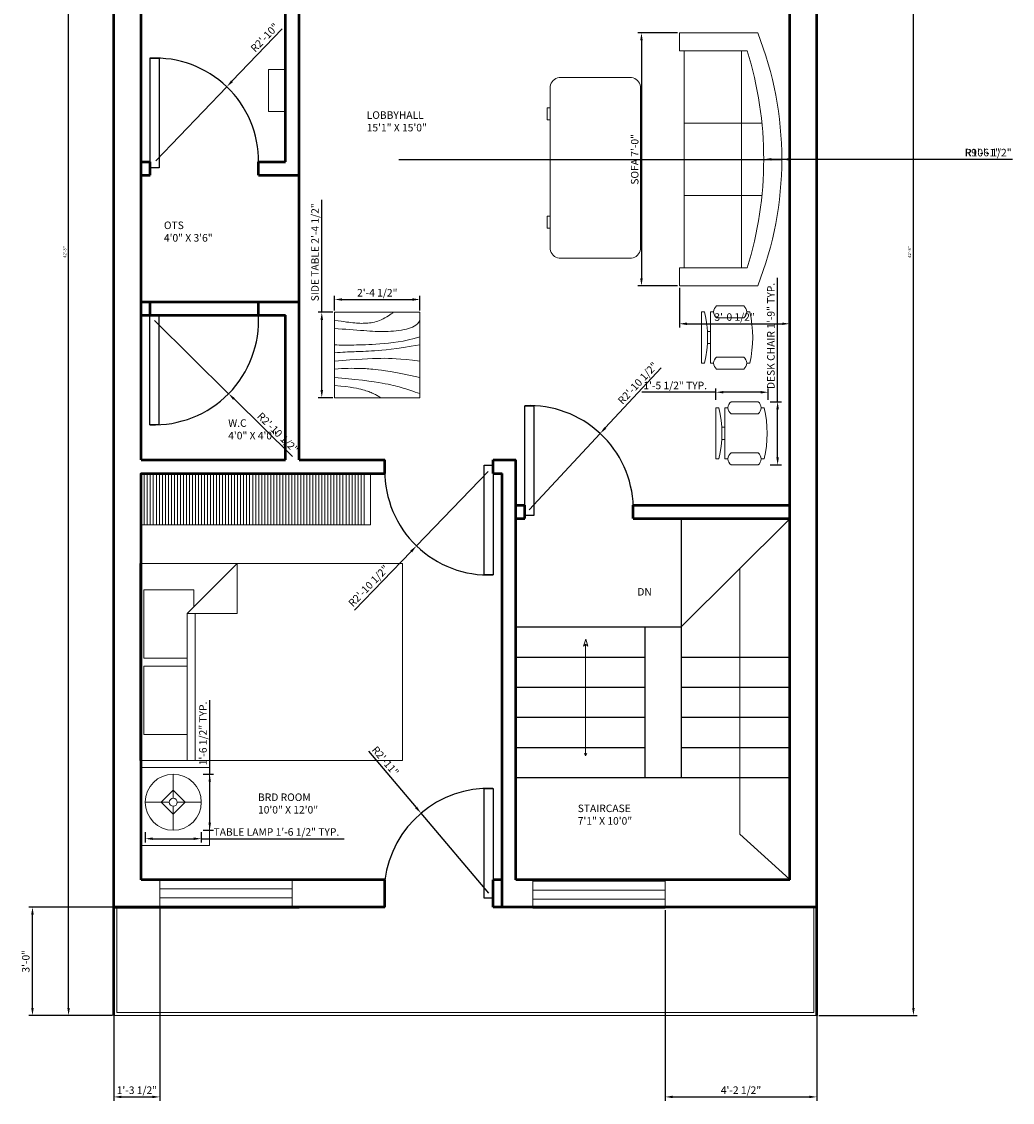
# Model space of a CAD drawing. Units: inches. Extents: x 210 to 950, y 0 to 561.
# Tile 4 of 5: x 621 to 950, y 8 to 366. Entities that reach past the tile are written whole.
import ezdxf

# ---------------------------------------------------------------- set-up
doc = ezdxf.new("R2010")
doc.units = ezdxf.units.IN
for name, color, linetype, lineweight in [('A-ANNO-DIMS', 2, 'Continuous', 18), ('A-ANNO-SYMB', 7, 'Continuous', 18), ('A-ANNO-TEXT', 7, 'Continuous', 18), ('A-AREA-IDEN', 7, 'Continuous', 18), ('A-DOOR', 4, 'Continuous', 25), ('A-FLOR-CASE', 8, 'Continuous', 20), ('A-FLOR-FIXT', 9, 'Continuous', 18), ('A-FLOR-HRAL', 7, 'Continuous', 18), ('A-FLOR-STRS', 7, 'Continuous', 25), ('A-FURN', 8, 'Continuous', 18), ('A-FURN-PATT', 9, 'Continuous', 13), ('A-GLAZ', 4, 'Continuous', 20), ('A-WALL', 7, 'Continuous', 50)]:
    doc.layers.add(name, color=color, linetype=linetype, lineweight=lineweight)
doc.styles.get("Standard").update_dxf_attribs({"font": 'arial.ttf'})
doc.dimstyles.new('ISO-25', dxfattribs={"dimtxt": 2.5, "dimasz": 2.5, "dimexe": 1.25, "dimexo": 0.625, "dimtad": 1, "dimtxsty": 'Standard', "dimcen": 2.5, "dimadec": 0, "dimazin": 0, "dimtfac": 1, "dimtmove": 0, "dimatfit": 3, "dimfxl": 1, "dimarcsym": 0})

# ---------------------------------------------------------------- blocks, each defined once
blk = doc.blocks.new('Bed - Queen')
for p, q in [((0, -80.00003), (0, 0)), ((0, 0), (59.99999, 0)), ((59.99999, 0), (59.99999, -80.00003)), ((7.99999, -1.2), (28.79998, -1.2)), ((7.99999, -14.4), (7.99999, -1.2)), ((28.79998, -1.2), (28.79998, -14.4)), ((31.19999, -1.2), (51.99999, -1.2)), ((31.19999, -14.4), (31.19999, -1.2)), ((51.99999, -1.2), (51.99999, -16.4)), ((0, -14.4), (44.8, -14.4)), ((59.99999, -29.6), (44.8, -14.4)), ((44.8, -14.4), (44.8, -29.6)), ((51.99999, -16.4), (46.79936, -16.4)), ((44.8, -16.8), (0, -16.8)), ((44.8, -29.6), (59.99999, -29.6)), ((59.99999, -80.00003), (0, -80.00003))]:
    blk.add_line(p, q)
blk = doc.blocks.new('Lamp - Table')
for p, q in [((0, 7), (0, 1)), ((0, 3), (-3, 0)), ((3, 0), (0, 3)), ((-1, 0), (-7, 0)), ((-3, 0), (0, -3)), ((0, -3), (3, 0)), ((1, 0), (7, 0)), ((0, -1), (0, -7))]:
    blk.add_line(p, q)
for radius in [7, 1]:
    blk.add_circle((0, 0), radius)
blk = doc.blocks.new('Sofa - Roundback 7 ft.')
for p, q in [((-12.00002, -32.4421), (-12.00003, -6.5971)), ((11.99997, -32.4421), (11.99998, -6.5971)), ((-36.000027, -34), (-36.000027, -11.4696)), ((-35.999844, -13.3819), (35.9998, -13.3819)), ((35.99998, -34), (35.99998, -11.4696)), ((-36.000027, -32.4421), (35.99998, -32.4421))]:
    blk.add_line(p, q)
for points in [[(-36.000027, -34), (-42.000027, -34), (-42.000027, -8)], [(41.99998, -8), (41.99998, -34), (35.99998, -34)]]:
    blk.add_lwpolyline(points)
for centre, radius, start, end in [((0, -114.25), 114.25, 68.43141, 111.5686), ((-0.00001, -127.1968), 121.1968, 72.72033, 107.2797)]:
    blk.add_arc(centre, radius, start, end)
blk = doc.blocks.new('Chair - Desk')
for p, q in [((-8.5, 0), (-8.5, -1)), ((-8.5, 0), (8.5, 0)), ((8.5, 0), (8.5, -1)), ((-8.5, -3), (-8.5, -4)), ((-8.5, -3), (8.5, -3)), ((-2, -3), (-2, -1.9355)), ((2, -1.9576), (2, -3)), ((8.5, -3), (8.5, -4)), ((-10.5, -5), (-10.5, -14)), ((-6.5, -14), (-6.5, -5)), ((6.5, -5), (6.5, -14)), ((10.5, -14), (10.5, -5)), ((-8.5, -15), (-8.5, -16)), ((8.5, -15), (8.5, -16))]:
    blk.add_line(p, q)
for centre, radius, start, end in [((0, 34.625), 36.625, 256.5803, 283.4197), ((-8.5, -6.5), 2.5, 36.8699, 143.1301), ((8.5, -6.5), 2.5, 36.8699, 143.1301), ((-8.5, -12.5), 2.5, 216.8699, 323.1301), ((8.5, -12.5), 2.5, 216.8699, 323.1301), ((0, 19.625), 36.625, 256.5803, 283.4197)]:
    blk.add_arc(centre, radius, start, end)
blk = doc.blocks.new('Desk - 30 x 60 in.')
for p, q in [((-26.999995, 0), (26.999995, 0)), ((-29.999995, -27), (-29.999995, -3)), ((29.999995, -3), (29.999995, -27)), ((26.999995, -30), (-26.999995, -30)), ((-20.000005, -30), (-20.000005, -31)), ((-20.000005, -31), (-16.000005, -31)), ((-16.000005, -31), (-16.000005, -30)), ((15.999995, -31), (15.999995, -30)), ((19.999995, -31), (15.999995, -31)), ((19.999995, -30), (19.999995, -31))]:
    blk.add_line(p, q)
for centre, start, end in [((-26.499995, -3.5), 98.1301, 171.8699), ((26.499995, -3.5), 8.130102, 81.8699), ((-26.499995, -26.5), 188.1301, 261.8699), ((26.499995, -26.5), 278.1301, 351.8699)]:
    blk.add_arc(centre, 3.535534, start, end)
blk = doc.blocks.new('Table - Square Woodgrain 42 x 42 in.')
blk.add_line((0, -42), (42, -42))
for points in [[(0, -4), (1.704, -4.2172), (3.2358, -4.4188), (4.615, -4.604), (5.8615, -4.7721), (6.9951, -4.9224), (8.0357, -5.0541), (9.0031, -5.1667), (9.9171, -5.2594), (10.7951, -5.3316), (11.6445, -5.3836), (12.4702, -5.4157), (13.277, -5.4283), (14.0698, -5.4217), (14.8535, -5.3964), (15.6331, -5.3526), (16.4133, -5.2908), (17.1986, -5.2103), (17.9913, -5.1062), (18.793, -4.9727), (19.6056, -4.8038), (20.4307, -4.5937), (21.2701, -4.3365), (22.1256, -4.0262), (22.9989, -3.6571), (23.888, -3.2272), (24.7756, -2.7516), (25.6408, -2.2491), (26.4624, -1.7387), (27.2195, -1.2395), (27.891, -0.7703), (28.456, -0.3501), (28.8934, 0.002)], [(0, -42), (0, 0), (42, 0), (42, -42)], [(0, -8), (1.8203, -8.1001), (3.6741, -8.2149), (5.5411, -8.3408), (7.4011, -8.4741), (9.2339, -8.6112), (11.0193, -8.7484), (12.7371, -8.8821), (14.3671, -9.0086), (15.8954, -9.1246), (17.3337, -9.2278), (18.6997, -9.3159), (20.0116, -9.387), (21.2871, -9.4389), (22.5442, -9.4696), (23.8008, -9.477), (25.0749, -9.459), (26.3791, -9.4137), (27.7049, -9.3403), (29.0383, -9.2382), (30.3655, -9.1068), (31.6728, -8.9455), (32.9461, -8.7535), (34.1717, -8.5304), (35.3358, -8.2756), (36.4268, -7.9863), (37.443, -7.6521), (38.3849, -7.2603), (39.253, -6.7986), (40.048, -6.2542), (40.7705, -5.6147), (41.421, -4.8674), (42, -4)], [(42, -12), (39.1784, -12.8621), (36.4519, -13.5654), (33.8246, -14.1294), (31.3004, -14.5731), (28.8832, -14.9161), (26.577, -15.1775), (24.3858, -15.3768), (22.3136, -15.5332), (20.3622, -15.6632), (18.5254, -15.7718), (16.7947, -15.8612), (15.1618, -15.9338), (13.6183, -15.9916), (12.1558, -16.0369), (10.7659, -16.0718), (9.4403, -16.0987), (8.1703, -16.1191), (6.9461, -16.1325), (5.7577, -16.1377), (4.595, -16.1335), (3.4479, -16.1188), (2.3064, -16.0924), (1.1604, -16.0532), (0, -16)], [(42, -16), (37.6529, -16.7365), (33.8802, -17.329), (30.6179, -17.7961), (27.8015, -18.1561), (25.3668, -18.4275), (23.2497, -18.6288), (21.3859, -18.7785), (19.7111, -18.8949), (18.1693, -18.9939), (16.7375, -19.0795), (15.401, -19.1534), (14.1449, -19.217), (12.9544, -19.2717), (11.8148, -19.3191), (10.7113, -19.3606), (9.6291, -19.3976), (8.5534, -19.4323), (7.47, -19.4689), (6.3643, -19.5122), (5.222, -19.5672), (4.0288, -19.6386), (2.7703, -19.7313), (1.4321, -19.8501), (0, -20)], [(0, -24), (3.9243, -23.6805), (7.4766, -23.4138), (10.6891, -23.1954), (13.5943, -23.0205), (16.2247, -22.8847), (18.6125, -22.7832), (20.7903, -22.7116), (22.7903, -22.6651), (24.6563, -22.642), (26.4764, -22.6507), (28.35, -22.7024), (30.3766, -22.8084), (32.6555, -22.98), (35.2861, -23.2283), (38.3678, -23.5645), (42, -24)], [(42, -32), (37.392, -31.017), (33.4585, -30.2231), (30.1291, -29.5949), (27.3334, -29.109), (25.0009, -28.742), (23.0612, -28.4707), (21.4439, -28.2716), (20.0786, -28.1215), (18.8998, -28.0002), (17.8609, -27.9014), (16.9206, -27.8219), (16.0371, -27.7588), (15.1691, -27.709), (14.2748, -27.6693), (13.3128, -27.6368), (12.2415, -27.6083), (11.0295, -27.5824), (9.6867, -27.5643), (8.233, -27.5608), (6.6884, -27.5787), (5.0728, -27.6248), (3.4062, -27.7058), (1.7086, -27.8286), (0, -28)], [(0, -32), (5.4026, -32.5358), (9.9494, -33.019), (13.7424, -33.4553), (16.8834, -33.8505), (19.4743, -34.2106), (21.6171, -34.5413), (23.4136, -34.8486), (24.9657, -35.1382), (26.3614, -35.4156), (27.6332, -35.6841), (28.7995, -35.9467), (29.8788, -36.2064), (30.8897, -36.4661), (31.8507, -36.7288), (32.7802, -36.9973), (33.6968, -37.2747), (34.6175, -37.5635), (35.5531, -37.8651), (36.5128, -38.1805), (37.506, -38.5108), (38.5421, -38.8568), (39.6302, -39.2197), (40.7797, -39.6004), (42, -40)], [(0, -36), (3.0098, -36.2857), (5.5354, -36.5643), (7.6368, -36.8359), (9.374, -37.1009), (10.807, -37.3597), (11.9957, -37.6126), (13.0002, -37.8599), (13.8804, -38.102), (14.6874, -38.3393), (15.4365, -38.5729), (16.1338, -38.8041), (16.7858, -39.0341), (17.3987, -39.264), (17.9787, -39.4952), (18.5322, -39.7288), (19.0655, -39.9662), (19.5832, -40.2081), (20.0842, -40.4544), (20.5657, -40.7046), (21.0249, -40.9581), (21.459, -41.2144), (21.8653, -41.4731), (22.2409, -41.7335), (22.5831, -41.9951)]]:
    blk.add_lwpolyline(points)
blk = doc.blocks.new('*D17')
at = {"layer": 'A-ANNO-DIMS', "color": 0, "lineweight": -2, "transparency": 16777216}
for p, q in [((651.28, 543.37), (635.61, 543.37)), ((636.86, 38.87), (636.86, 540.87)), ((651.28, 36.37), (635.61, 36.37))]:
    blk.add_line(p, q, dxfattribs=at)
at = {"layer": 'A-ANNO-DIMS', "color": 0, "transparency": 16777216}
for points in [[(636.44, 540.87), (637.27, 540.87), (636.86, 543.37)], [(636.44, 38.87), (637.27, 38.87), (636.86, 36.37)]]:
    blk.add_solid(points, dxfattribs=at)
at = {"layer": 'Defpoints', "color": 0, "transparency": 16777216}
for p in [(636.86, 543.37), (651.91, 543.37), (651.91, 36.37)]:
    blk.add_point(p, dxfattribs=at)
at = {"layer": 'A-ANNO-DIMS', "color": 0, "transparency": 16777216, "insert": (635.72, 289.87), "char_height": 1, "attachment_point": 5, "rotation": 90}
blk.add_mtext('42\'-3"', dxfattribs=at)
blk = doc.blocks.new('*D19')
at = {"layer": 'A-ANNO-DIMS', "color": 0, "lineweight": -2, "transparency": 16777216}
for p, q in [((886.03, 543.37), (918.72, 543.37)), ((917.47, 38.87), (917.47, 540.87)), ((886.03, 36.37), (918.72, 36.37))]:
    blk.add_line(p, q, dxfattribs=at)
at = {"layer": 'A-ANNO-DIMS', "color": 0, "transparency": 16777216}
for points in [[(917.05, 540.87), (917.89, 540.87), (917.47, 543.37)], [(917.05, 38.87), (917.89, 38.87), (917.47, 36.37)]]:
    blk.add_solid(points, dxfattribs=at)
at = {"layer": 'Defpoints', "color": 0, "transparency": 16777216}
for p in [(885.41, 543.37), (917.47, 543.37), (885.41, 36.37)]:
    blk.add_point(p, dxfattribs=at)
at = {"layer": 'A-ANNO-DIMS', "color": 0, "transparency": 16777216, "insert": (916.33, 289.87), "char_height": 1, "attachment_point": 5, "rotation": 90}
blk.add_mtext('42\'-3"', dxfattribs=at)
blk = doc.blocks.new('WIN-44IN-DEEP-FRAME')
for p, q in [((0, 0), (0, 9)), ((0, 9), (43.89, 9)), ((43.89, 9), (43.89, 0)), ((43.89, 6), (0, 6)), ((0, 3), (43.89, 3)), ((43.89, 0), (0, 0))]:
    blk.add_line(p, q)
blk = doc.blocks.new('DOOR-LEAF-36IN')
blk.add_lwpolyline([(0, 0), (0, -2.99), (-36.41, -2.99), (-36.41, 0)], close=True)
blk = doc.blocks.new('*D26')
at = {"layer": 'A-ANNO-DIMS', "color": 0, "lineweight": -2, "transparency": 16777216}
for p, q in [((662.31, 97.23), (662.31, 93.81)), ((680.94, 97.23), (680.94, 93.81)), ((664.81, 95.06), (678.44, 95.06)), ((680.94, 95.06), (728.34, 95.06))]:
    blk.add_line(p, q, dxfattribs=at)
at = {"layer": 'A-ANNO-DIMS', "color": 0, "transparency": 16777216}
for points in [[(664.81, 95.48), (664.81, 94.64), (662.31, 95.06)], [(678.44, 95.48), (678.44, 94.64), (680.94, 95.06)]]:
    blk.add_solid(points, dxfattribs=at)
at = {"layer": 'Defpoints', "color": 0, "transparency": 16777216}
for p in [(662.31, 97.85), (680.94, 97.85), (680.94, 95.06)]:
    blk.add_point(p, dxfattribs=at)
at = {"layer": 'A-ANNO-DIMS', "color": 0, "transparency": 16777216, "insert": (705.89, 96.98), "char_height": 2.5, "attachment_point": 5}
blk.add_mtext('TABLE LAMP 1\'-6 1/2" TYP.', dxfattribs=at)
blk = doc.blocks.new('*D27')
at = {"layer": 'A-ANNO-DIMS', "color": 0, "lineweight": -2, "transparency": 16777216}
for p, q in [((683.74, 116.48), (683.74, 141.06)), ((681.57, 116.48), (684.99, 116.48)), ((683.74, 100.35), (683.74, 113.98)), ((681.57, 97.85), (684.99, 97.85))]:
    blk.add_line(p, q, dxfattribs=at)
at = {"layer": 'A-ANNO-DIMS', "color": 0, "transparency": 16777216}
for points in [[(683.32, 113.98), (684.15, 113.98), (683.74, 116.48)], [(683.32, 100.35), (684.15, 100.35), (683.74, 97.85)]]:
    blk.add_solid(points, dxfattribs=at)
at = {"layer": 'Defpoints', "color": 0, "transparency": 16777216}
for p in [(680.94, 116.48), (683.74, 116.48), (680.94, 97.85)]:
    blk.add_point(p, dxfattribs=at)
at = {"layer": 'A-ANNO-DIMS', "color": 0, "transparency": 16777216, "insert": (681.82, 130.02), "char_height": 2.5, "attachment_point": 5, "rotation": 90}
blk.add_mtext('1\'-6 1/2" TYP.', dxfattribs=at)
blk = doc.blocks.new('*D28')
at = {"layer": 'A-ANNO-DIMS', "color": 0, "lineweight": -2, "transparency": 16777216}
for p, q in [((872.36, 240.17), (872.36, 281.35)), ((869.84, 240.17), (873.61, 240.17)), ((872.36, 221.67), (872.36, 237.67)), ((869.84, 219.17), (873.61, 219.17))]:
    blk.add_line(p, q, dxfattribs=at)
at = {"layer": 'A-ANNO-DIMS', "color": 0, "transparency": 16777216}
for points in [[(871.95, 237.67), (872.78, 237.67), (872.36, 240.17)], [(871.95, 221.67), (872.78, 221.67), (872.36, 219.17)]]:
    blk.add_solid(points, dxfattribs=at)
at = {"layer": 'Defpoints', "color": 0, "transparency": 16777216}
for p in [(869.21, 240.17), (872.36, 240.17), (869.21, 219.17)]:
    blk.add_point(p, dxfattribs=at)
at = {"layer": 'A-ANNO-DIMS', "color": 0, "transparency": 16777216, "insert": (870.45, 262.01), "char_height": 2.5, "attachment_point": 5, "rotation": 90}
blk.add_mtext('DESK CHAIR 1\'-9" TYP.', dxfattribs=at)
blk = doc.blocks.new('*D29')
at = {"layer": 'A-ANNO-DIMS', "color": 0, "lineweight": -2, "transparency": 16777216}
for p, q in [((851.88, 240.79), (851.88, 244.57)), ((869.21, 240.79), (869.21, 244.57)), ((851.88, 243.32), (827.3, 243.32)), ((866.71, 243.32), (854.38, 243.32))]:
    blk.add_line(p, q, dxfattribs=at)
at = {"layer": 'A-ANNO-DIMS', "color": 0, "transparency": 16777216}
for points in [[(854.38, 243.73), (854.38, 242.9), (851.88, 243.32)], [(866.71, 243.73), (866.71, 242.9), (869.21, 243.32)]]:
    blk.add_solid(points, dxfattribs=at)
at = {"layer": 'Defpoints', "color": 0, "transparency": 16777216}
for p in [(851.88, 243.32), (851.88, 240.17), (869.21, 240.17)]:
    blk.add_point(p, dxfattribs=at)
at = {"layer": 'A-ANNO-DIMS', "color": 0, "transparency": 16777216, "insert": (838.34, 245.24), "char_height": 2.5, "attachment_point": 5}
blk.add_mtext('1\'-5 1/2" TYP.', dxfattribs=at)
blk = doc.blocks.new('*D34')
at = {"layer": 'A-ANNO-DIMS', "color": 0, "lineweight": -2, "transparency": 16777216}
for p, q in [((720.95, 269.86), (720.95, 307.23)), ((724.58, 269.86), (719.7, 269.86)), ((720.95, 244.01), (720.95, 267.36)), ((724.58, 241.51), (719.7, 241.51))]:
    blk.add_line(p, q, dxfattribs=at)
at = {"layer": 'A-ANNO-DIMS', "color": 0, "transparency": 16777216}
for points in [[(720.53, 267.36), (721.37, 267.36), (720.95, 269.86)], [(720.53, 244.01), (721.37, 244.01), (720.95, 241.51)]]:
    blk.add_solid(points, dxfattribs=at)
at = {"layer": 'Defpoints', "color": 0, "transparency": 16777216}
for p in [(720.95, 269.86), (725.2, 269.86), (725.2, 241.51)]:
    blk.add_point(p, dxfattribs=at)
at = {"layer": 'A-ANNO-DIMS', "color": 0, "transparency": 16777216, "insert": (719.03, 289.79), "char_height": 2.5, "attachment_point": 5, "rotation": 90}
blk.add_mtext('SIDE TABLE 2\'-4 1/2"', dxfattribs=at)
blk = doc.blocks.new('*D35')
at = {"layer": 'A-ANNO-DIMS', "color": 0, "lineweight": -2, "transparency": 16777216}
for p, q in [((725.2, 270.49), (725.2, 275.36)), ((727.7, 274.11), (751.05, 274.11)), ((753.55, 270.49), (753.55, 275.36))]:
    blk.add_line(p, q, dxfattribs=at)
at = {"layer": 'A-ANNO-DIMS', "color": 0, "transparency": 16777216}
for points in [[(727.7, 274.53), (727.7, 273.7), (725.2, 274.11)], [(751.05, 274.53), (751.05, 273.7), (753.55, 274.11)]]:
    blk.add_solid(points, dxfattribs=at)
at = {"layer": 'Defpoints', "color": 0, "transparency": 16777216}
for p in [(753.55, 274.11), (725.2, 269.86), (753.55, 269.86)]:
    blk.add_point(p, dxfattribs=at)
at = {"layer": 'A-ANNO-DIMS', "color": 0, "transparency": 16777216, "insert": (739.38, 276.03), "char_height": 2.5, "attachment_point": 5}
blk.add_mtext('2\'-4 1/2"', dxfattribs=at)
blk = doc.blocks.new('*D40')
at = {"layer": 'A-ANNO-DIMS', "color": 0, "lineweight": -2, "transparency": 16777216}
for p, q in [((839.11, 362.65), (825.89, 362.65)), ((827.14, 360.15), (827.14, 281.15)), ((839.11, 278.65), (825.89, 278.65))]:
    blk.add_line(p, q, dxfattribs=at)
at = {"layer": 'A-ANNO-DIMS', "color": 0, "transparency": 16777216}
for points in [[(826.72, 360.15), (827.55, 360.15), (827.14, 362.65)], [(826.72, 281.15), (827.55, 281.15), (827.14, 278.65)]]:
    blk.add_solid(points, dxfattribs=at)
at = {"layer": 'Defpoints', "color": 0, "transparency": 16777216}
for p in [(839.74, 362.65), (827.14, 278.65), (839.74, 278.65)]:
    blk.add_point(p, dxfattribs=at)
at = {"layer": 'A-ANNO-DIMS', "color": 0, "transparency": 16777216, "insert": (825.22, 320.65), "char_height": 2.5, "attachment_point": 5, "rotation": 90}
blk.add_mtext('SOFA 7\'-0"', dxfattribs=at)
blk = doc.blocks.new('*D41')
at = {"layer": 'A-ANNO-DIMS', "color": 0, "lineweight": -2, "transparency": 16777216}
for p, q in [((839.74, 278.03), (839.74, 264.8)), ((876.4, 278.03), (876.4, 264.8)), ((842.24, 266.05), (873.9, 266.05))]:
    blk.add_line(p, q, dxfattribs=at)
at = {"layer": 'A-ANNO-DIMS', "color": 0, "transparency": 16777216}
for points in [[(842.24, 266.47), (842.24, 265.64), (839.74, 266.05)], [(873.9, 266.47), (873.9, 265.64), (876.4, 266.05)]]:
    blk.add_solid(points, dxfattribs=at)
at = {"layer": 'Defpoints', "color": 0, "transparency": 16777216}
for p in [(839.74, 278.65), (876.4, 278.65), (876.4, 266.05)]:
    blk.add_point(p, dxfattribs=at)
at = {"layer": 'A-ANNO-DIMS', "color": 0, "transparency": 16777216, "insert": (858.07, 267.97), "char_height": 2.5, "attachment_point": 5}
blk.add_mtext('3\'-0 1/2"', dxfattribs=at)
blk = doc.blocks.new('*D48')
at = {"layer": 'A-ANNO-DIMS', "color": 0, "lineweight": -2, "transparency": 16777216}
for p, q in [((651.28, 72.37), (623.61, 72.37)), ((624.86, 38.87), (624.86, 69.87)), ((651.28, 36.37), (623.61, 36.37))]:
    blk.add_line(p, q, dxfattribs=at)
at = {"layer": 'A-ANNO-DIMS', "color": 0, "transparency": 16777216}
for points in [[(624.44, 69.87), (625.27, 69.87), (624.86, 72.37)], [(624.44, 38.87), (625.27, 38.87), (624.86, 36.37)]]:
    blk.add_solid(points, dxfattribs=at)
at = {"layer": 'Defpoints', "color": 0, "transparency": 16777216}
for p in [(624.86, 72.37), (651.91, 72.37), (651.91, 36.37)]:
    blk.add_point(p, dxfattribs=at)
at = {"layer": 'A-ANNO-DIMS', "color": 0, "transparency": 16777216, "insert": (622.96, 54.37), "char_height": 2.5, "attachment_point": 5, "rotation": 90}
blk.add_mtext('3\'-0"', dxfattribs=at)
blk = doc.blocks.new('*D50')
at = {"layer": 'A-ANNO-DIMS', "color": 0, "lineweight": -2, "transparency": 16777216}
for p, q in [((651.91, 71.74), (651.91, 8.07)), ((667.18, 71.76), (667.18, 8.07)), ((654.41, 9.32), (664.68, 9.32))]:
    blk.add_line(p, q, dxfattribs=at)
at = {"layer": 'A-ANNO-DIMS', "color": 0, "transparency": 16777216}
for points in [[(654.41, 9.73), (654.41, 8.9), (651.91, 9.32)], [(664.68, 9.73), (664.68, 8.9), (667.18, 9.32)]]:
    blk.add_solid(points, dxfattribs=at)
at = {"layer": 'Defpoints', "color": 0, "transparency": 16777216}
for p in [(651.91, 72.37), (667.18, 72.39), (667.18, 9.32)]:
    blk.add_point(p, dxfattribs=at)
at = {"layer": 'A-ANNO-DIMS', "color": 0, "transparency": 16777216, "insert": (659.54, 11.23), "char_height": 2.5, "attachment_point": 5}
blk.add_mtext('1\'-3 1/2"', dxfattribs=at)
blk = doc.blocks.new('*D51')
at = {"layer": 'A-ANNO-DIMS', "color": 0, "lineweight": -2, "transparency": 16777216}
for p, q in [((835, 71.37), (835, 8.07)), ((885.41, 71.74), (885.41, 8.07)), ((837.5, 9.32), (882.91, 9.32))]:
    blk.add_line(p, q, dxfattribs=at)
at = {"layer": 'A-ANNO-DIMS', "color": 0, "transparency": 16777216}
for points in [[(837.5, 9.73), (837.5, 8.9), (835, 9.32)], [(882.91, 9.73), (882.91, 8.9), (885.41, 9.32)]]:
    blk.add_solid(points, dxfattribs=at)
at = {"layer": 'Defpoints', "color": 0, "transparency": 16777216}
for p in [(835, 72), (885.41, 72.37), (885.41, 9.32)]:
    blk.add_point(p, dxfattribs=at)
at = {"layer": 'A-ANNO-DIMS', "color": 0, "transparency": 16777216, "insert": (860.2, 11.23), "char_height": 2.5, "attachment_point": 5}
blk.add_mtext('4\'-2 1/2"', dxfattribs=at)
blk = doc.blocks.new('*D58')
at = {"layer": 'A-ANNO-DIMS', "color": 0, "lineweight": -2, "transparency": 16777216}
for p, q in [((736.45, 124.09), (752.31, 105.42)), ((776.45, 77), (753.92, 103.52))]:
    blk.add_line(p, q, dxfattribs=at)
at = {"layer": 'A-ANNO-DIMS', "color": 0, "transparency": 16777216}
blk.add_solid([(752.62, 105.69), (751.99, 105.15), (753.92, 103.52)], dxfattribs=at)
at = {"layer": 'Defpoints', "color": 0, "transparency": 16777216}
for p in [(753.92, 103.52), (776.45, 77)]:
    blk.add_point(p, dxfattribs=at)
at = {"layer": 'A-ANNO-DIMS', "color": 0, "transparency": 16777216, "insert": (741.84, 120.64), "char_height": 2.5, "attachment_point": 5, "rotation": 310.3522}
blk.add_mtext('R2\'-11"', dxfattribs=at)
blk = doc.blocks.new('*D59')
at = {"layer": 'A-ANNO-DIMS', "color": 0, "lineweight": -2, "transparency": 16777216}
for p, q in [((665.34, 267.11), (690.01, 242.83)), ((711.25, 221.93), (691.8, 241.08))]:
    blk.add_line(p, q, dxfattribs=at)
at = {"layer": 'A-ANNO-DIMS', "color": 0, "transparency": 16777216}
blk.add_solid([(692.09, 241.37), (691.5, 240.78), (690.01, 242.83)], dxfattribs=at)
at = {"layer": 'Defpoints', "color": 0, "transparency": 16777216}
for p in [(665.34, 267.11), (690.01, 242.83)]:
    blk.add_point(p, dxfattribs=at)
at = {"layer": 'A-ANNO-DIMS', "color": 0, "transparency": 16777216, "insert": (706.16, 229.63), "char_height": 2.5, "attachment_point": 5, "rotation": 315.4554}
blk.add_mtext('R2\'-10 1/2"', dxfattribs=at)
blk = doc.blocks.new('*D60')
at = {"layer": 'A-ANNO-DIMS', "color": 0, "lineweight": -2, "transparency": 16777216}
for p, q in [((833.69, 251.41), (815.13, 231.45)), ((789.89, 204.32), (813.42, 229.62))]:
    blk.add_line(p, q, dxfattribs=at)
at = {"layer": 'A-ANNO-DIMS', "color": 0, "transparency": 16777216}
blk.add_solid([(814.82, 231.73), (815.43, 231.17), (813.42, 229.62)], dxfattribs=at)
at = {"layer": 'Defpoints', "color": 0, "transparency": 16777216}
for p in [(813.42, 229.62), (789.89, 204.32)]:
    blk.add_point(p, dxfattribs=at)
at = {"layer": 'A-ANNO-DIMS', "color": 0, "transparency": 16777216, "insert": (826.14, 246.11), "char_height": 2.5, "attachment_point": 5, "rotation": 47.0742}
blk.add_mtext('R2\'-10 1/2"', dxfattribs=at)
blk = doc.blocks.new('*D61')
at = {"layer": 'A-ANNO-DIMS', "color": 0, "lineweight": -2, "transparency": 16777216}
for p, q in [((776.26, 217), (752.41, 192.28)), ((731.83, 170.95), (750.68, 190.48))]:
    blk.add_line(p, q, dxfattribs=at)
at = {"layer": 'A-ANNO-DIMS', "color": 0, "transparency": 16777216}
blk.add_solid([(750.38, 190.77), (750.97, 190.19), (752.41, 192.28)], dxfattribs=at)
at = {"layer": 'Defpoints', "color": 0, "transparency": 16777216}
for p in [(776.26, 217), (752.41, 192.28)]:
    blk.add_point(p, dxfattribs=at)
at = {"layer": 'A-ANNO-DIMS', "color": 0, "transparency": 16777216, "insert": (736.72, 178.78), "char_height": 2.5, "attachment_point": 5, "rotation": 46.0238}
blk.add_mtext('R2\'-10 1/2"', dxfattribs=at)
blk = doc.blocks.new('*D63')
at = {"layer": 'A-ANNO-DIMS', "color": 0, "lineweight": -2, "transparency": 16777216}
for p, q in [((707.81, 363.95), (691.13, 346.56)), ((665.79, 320.12), (689.4, 344.76))]:
    blk.add_line(p, q, dxfattribs=at)
at = {"layer": 'A-ANNO-DIMS', "color": 0, "transparency": 16777216}
blk.add_solid([(690.83, 346.85), (691.44, 346.28), (689.4, 344.76)], dxfattribs=at)
at = {"layer": 'Defpoints', "color": 0, "transparency": 16777216}
for p in [(689.4, 344.76), (665.79, 320.12)]:
    blk.add_point(p, dxfattribs=at)
at = {"layer": 'A-ANNO-DIMS', "color": 0, "transparency": 16777216, "insert": (702.2, 360.86), "char_height": 2.5, "attachment_point": 5, "rotation": 46.2105}
blk.add_mtext('R2\'-10"', dxfattribs=at)
blk = doc.blocks.new('*D67')
at = {"layer": 'A-ANNO-DIMS', "color": 0, "lineweight": -2, "transparency": 16777216}
for p, q in [((746.54, 320.65), (867.74, 320.65)), ((946.57, 320.65), (870.24, 320.65))]:
    blk.add_line(p, q, dxfattribs=at)
at = {"layer": 'A-ANNO-DIMS', "color": 0, "transparency": 16777216}
blk.add_solid([(870.24, 321.07), (870.24, 320.24), (867.74, 320.65)], dxfattribs=at)
at = {"layer": 'Defpoints', "color": 0, "transparency": 16777216}
for p in [(746.54, 320.65), (867.74, 320.65)]:
    blk.add_point(p, dxfattribs=at)
at = {"layer": 'A-ANNO-DIMS', "color": 0, "transparency": 16777216, "insert": (940.45, 322.56), "char_height": 2.5, "attachment_point": 5}
blk.add_mtext('R10\'-1"', dxfattribs=at)
blk = doc.blocks.new('*D68')
at = {"layer": 'A-ANNO-DIMS', "color": 0, "lineweight": -2, "transparency": 16777216}
for p, q in [((759.49, 320.65), (873.74, 320.65)), ((950.34, 320.65), (876.24, 320.65))]:
    blk.add_line(p, q, dxfattribs=at)
at = {"layer": 'A-ANNO-DIMS', "color": 0, "transparency": 16777216}
blk.add_solid([(876.24, 321.07), (876.24, 320.24), (873.74, 320.65)], dxfattribs=at)
at = {"layer": 'Defpoints', "color": 0, "transparency": 16777216}
for p in [(759.49, 320.65), (873.74, 320.65)]:
    blk.add_point(p, dxfattribs=at)
at = {"layer": 'A-ANNO-DIMS', "color": 0, "transparency": 16777216, "insert": (942.29, 322.57), "char_height": 2.5, "attachment_point": 5, "rotation": 0}
blk.add_mtext('R9\'-6 1/2"', dxfattribs=at)

msp = doc.modelspace()

# ---------------------------------------------------------------- hatches: boundary and pattern name
at = {"layer": 'A-FURN-PATT'}
h = msp.add_hatch(dxfattribs=at)
h.set_pattern_fill('ANSI31', color=256, scale=0.314961, angle=45, style=0)
h.paths.add_polyline_path([(660.82, 199.32), (735.38, 199.32), (735.38, 216.37), (660.82, 216.37)])

# ---------------------------------------------------------------- linework, layer by layer
at = {"layer": 'A-ANNO-SYMB'}
for p, q in [((859.81, 96.57), (859.81, 184.76)), ((808.64, 161.32), (807.84, 158.95)), ((807.84, 158.95), (808.59, 159.57)), ((808.56, 123.16), (808.56, 159.7)), ((808.56, 159.7), (809.29, 159.05)), ((809.29, 159.05), (808.64, 161.32)), ((808.54, 122.61), (808.17, 123.37)), ((808.17, 123.37), (808.56, 123.17)), ((808.94, 123.39), (808.54, 122.61)), ((808.55, 123.16), (808.94, 123.39)), ((876.27, 81.58), (859.81, 96.57))]:
    msp.add_line(p, q, dxfattribs=at)
at = {"layer": 'A-DOOR'}
for centre, radius, start, end in [((665.79, 320.12), 34.13, 359.2311, 93.1904), ((665.34, 267.11), 34.61, 267.5759, 3.336), ((789.89, 204.32), 34.55, 1.6517, 92.4945), ((776.26, 217), 34.35, 179.4037, 272.6424), ((776.45, 77), 34.8, 87.7468, 172.9571)]:
    msp.add_arc(centre, radius, start, end, dxfattribs=at)
at = {"layer": 'A-FLOR-CASE'}
msp.add_lwpolyline([(660.78, 216.43), (737.19, 216.43), (737.19, 199.29), (660.78, 199.29)], close=True, dxfattribs=at)
at = {"layer": 'A-FLOR-FIXT'}
msp.add_lwpolyline([(708.91, 350.53), (703.27, 350.53), (703.27, 336.56), (708.91, 336.56)], close=True, dxfattribs=at)
at = {"layer": 'A-FLOR-HRAL'}
for p, q in [((652.91, 37.37), (652.91, 72.37)), ((884.41, 37.37), (884.41, 72.37)), ((885.41, 36.37), (651.91, 36.37)), ((884.41, 37.37), (652.91, 37.37)), ((885.41, 36.37), (777.91, 36.37))]:
    msp.add_line(p, q, dxfattribs=at)
at = {"layer": 'A-FLOR-STRS'}
for p, q in [((840.14, 165.19), (876.28, 201.15)), ((840.41, 115.37), (840.41, 201.37)), ((785.41, 165.37), (840.41, 165.37)), ((828.41, 115.37), (828.41, 165.37)), ((785.41, 155.37), (828.41, 155.37)), ((840.41, 155.37), (876.41, 155.37)), ((785.41, 145.37), (828.41, 145.37)), ((840.41, 145.37), (876.41, 145.37)), ((785.41, 135.37), (828.41, 135.37)), ((840.41, 135.37), (876.41, 135.37)), ((785.41, 125.37), (828.41, 125.37)), ((840.41, 125.37), (876.41, 125.37)), ((785.41, 115.37), (876.41, 115.37)), ((876.27, 81.42), (862.23, 81.42))]:
    msp.add_line(p, q, dxfattribs=at)
at = {"layer": 'A-FURN'}
msp.add_lwpolyline([(660.87, 118.7), (683.71, 118.7), (683.71, 92.84), (660.87, 92.84)], close=True, dxfattribs=at)
at = {"layer": 'A-WALL'}
for p, q in [((651.91, 36.37), (651.91, 543.37)), ((885.41, 36.37), (885.41, 543.37)), ((660.91, 315.37), (660.91, 385.87)), ((708.91, 319.87), (708.91, 385.87)), ((713.41, 315.37), (713.41, 385.87)), ((713.41, 268.87), (713.41, 385.87)), ((713.41, 220.87), (713.41, 385.87)), ((876.41, 81.37), (876.41, 385.87)), ((660.91, 319.87), (663.91, 319.87)), ((663.91, 315.37), (663.91, 319.87)), ((699.91, 315.37), (699.91, 319.87)), ((699.91, 319.87), (708.91, 319.87)), ((660.91, 315.37), (663.91, 315.37)), ((660.91, 268.87), (660.91, 315.37)), ((699.91, 315.37), (713.41, 315.37)), ((660.91, 273.37), (713.41, 273.37)), ((663.91, 268.87), (663.91, 273.37)), ((699.91, 268.87), (699.91, 273.37)), ((660.91, 268.87), (708.91, 268.87)), ((660.91, 220.87), (660.91, 268.87)), ((708.91, 220.87), (708.91, 268.87)), ((660.91, 220.87), (708.91, 220.87)), ((713.41, 220.87), (741.91, 220.87)), ((741.91, 216.37), (741.91, 220.87)), ((777.91, 216.37), (777.91, 220.87)), ((777.91, 220.87), (785.41, 220.87)), ((785.41, 81.37), (785.41, 220.87)), ((660.91, 81.37), (660.91, 216.37)), ((660.91, 216.37), (741.91, 216.37)), ((777.91, 216.37), (780.91, 216.37)), ((780.91, 72.37), (780.91, 216.37)), ((785.41, 205.87), (788.41, 205.87)), ((788.41, 201.37), (788.41, 205.87)), ((824.41, 201.37), (824.41, 205.87)), ((824.41, 205.87), (876.41, 205.87)), ((785.41, 201.37), (788.41, 201.37)), ((824.41, 201.37), (876.41, 201.37)), ((741.91, 81.37), (660.91, 81.37)), ((741.91, 72.37), (741.91, 81.37)), ((777.91, 72.37), (777.91, 81.37)), ((780.91, 81.37), (777.91, 81.37)), ((876.41, 81.37), (785.41, 81.37)), ((651.91, 72.37), (713.41, 72.37)), ((741.91, 72.37), (651.91, 72.37)), ((885.41, 72.37), (777.91, 72.37))]:
    msp.add_line(p, q, dxfattribs=at)

# ---------------------------------------------------------------- block references
at = {"layer": 'A-DOOR'}
for p, rotation in [((666.92, 317.82), 270), ((666.88, 232.53), 270), ((791.39, 202.44), 270), ((777.83, 182.68), 270.0000000000003), ((777.83, 75.36), 270)]:
    msp.add_blockref('DOOR-LEAF-36IN', p, dxfattribs=dict(at, rotation=rotation))
at = {"layer": 'A-FURN'}
for name, p, rotation in [('Sofa - Roundback 7 ft.', (873.74, 320.65), 270), ('Desk - 30 x 60 in.', (826.79, 317.8), 270), ('Chair - Desk', (847.1, 261.51), 90), ('Chair - Desk', (851.88, 229.67), 90)]:
    msp.add_blockref(name, p, dxfattribs=dict(at, rotation=rotation))
for name, p, xscale, yscale, zscale in [('Table - Square Woodgrain 42 x 42 in.', (725.2, 269.86), 0.6750077513191393, 0.6750077513191393, 0.6750077513191393), ('Lamp - Table', (671.63, 107.17), 1.330786106251803, 1.330786106251803, 1.330786106251803)]:
    msp.add_blockref(name, p, dxfattribs=dict(at, xscale=xscale, yscale=yscale, zscale=zscale))
at = {"layer": 'A-FURN', "xscale": 1.090825566177695, "yscale": 1.090825566177695, "zscale": 1.090825566177695, "rotation": 90}
msp.add_blockref('Bed - Queen', (660.55, 120.98), dxfattribs=at)
at = {"layer": 'A-GLAZ'}
for p in [(667.18, 72.39), (791.1, 72)]:
    msp.add_blockref('WIN-44IN-DEEP-FRAME', p, dxfattribs=at)

# ---------------------------------------------------------------- texts
at = {"layer": 'A-ANNO-TEXT', "insert": (825.77, 178.3), "char_height": 2.5, "attachment_point": 1}
msp.add_mtext_dynamic_manual_height_columns('DN', width=6.5056, gutter_width=12.5, heights=[0], dxfattribs=at)
at = {"layer": 'A-AREA-IDEN', "char_height": 2.5, "attachment_point": 1}
for s, width, insert in [('LOBBYHALL\\P15\'1" X 15\'0"', 68.746, (735.88, 336.6)), ('OTS\\P4\'0" X 3\'6"', 25.7686, (668.52, 300)), ('W.C\\P4\'0" X 4\'0"', 30.5882, (689.87, 234.33)), ('BRD ROOM\\P10\'0" X 12\'0"', 23.2991, (699.77, 110.09)), ('STAIRCASE\\P7\'1" X 10\'0"', 31.1205, (805.97, 106.39))]:
    msp.add_mtext_dynamic_manual_height_columns(s, width=width, gutter_width=12.5, heights=[0], dxfattribs=dict(at, insert=insert))

# ---------------------------------------------------------------- dimensions: what is measured, and where the dimension line sits
at = {"layer": 'A-ANNO-DIMS'}
for base, p1, p2, override, picture, middle in [((636.86, 543.37), (651.91, 36.37), (651.91, 543.37), {"dimtxt": 1, "dimdec": 0, "dimlunit": 3, "dimclrd": 0, "dimclre": 0, "dimclrt": 0, "dimtdec": 0}, '*D17', (635.72, 289.87)), ((917.47, 543.37), (885.41, 36.37), (885.41, 543.37), {"dimtxt": 1, "dimdec": 0, "dimlunit": 3, "dimclrd": 0, "dimclre": 0, "dimclrt": 0, "dimtdec": 0}, '*D19', (916.33, 289.87)), ((624.86, 72.37), (651.91, 36.37), (651.91, 72.37), {"dimdec": 1, "dimlfac": 1, "dimrnd": 0, "dimzin": 1, "dimdsep": 46, "dimlunit": 4, "dimfrac": 2}, '*D48', (622.96, 54.37))]:
    dim = msp.add_linear_dim(base=base, p1=p1, p2=p2, angle=90, dimstyle='ISO-25', override=override, dxfattribs=at)
    dim.commit()
    dim.dimension.update_dxf_attribs({"geometry": picture, "text_midpoint": middle})
for center, mpoint, picture, middle in [((665.79, 320.12), (689.4, 344.76), '*D63', (703.57, 359.54)), ((746.54, 320.65), (867.74, 320.65), '*D67', (940.45, 320.65)), ((759.485651, 320.65399), (873.735651, 320.654), '*D68', (942.285651, 320.654006)), ((665.34, 267.11), (690.01, 242.83), '*D59', (704.82, 228.26)), ((789.89, 204.32), (813.42, 229.62), '*D60', (827.54, 244.8)), ((776.2638, 217.0038), (752.411, 192.283), '*D61', (738.0994, 177.4505)), ((776.45, 77), (753.92, 103.52), '*D58', (740.41, 119.43))]:
    dim = msp.add_radius_dim(center=center, mpoint=mpoint, dimstyle='ISO-25', override={"dimdec": 1, "dimlfac": 1, "dimrnd": 0, "dimzin": 1, "dimdsep": 46, "dimlunit": 4, "dimfrac": 2}, dxfattribs=at)
    dim.commit()
    dim.dimension.update_dxf_attribs({"geometry": picture, "text_midpoint": middle, "dimtype": 164})
for base, p1, p2, angle, text, picture, middle in [((827.14, 278.65), (839.74, 362.65), (839.74, 278.65), 270, 'SOFA <>', '*D40', (825.22, 320.65)), ((720.9485, 269.8601), (725.2012, 241.5084), (725.2012, 269.8601), 90, 'SIDE TABLE <>', '*D34', (719.0309, 289.7927)), ((872.36, 240.17), (869.21, 219.17), (869.21, 240.17), 90, 'DESK CHAIR <> TYP.', '*D28', (870.45, 262.01)), ((851.88, 243.32), (869.21, 240.17), (851.88, 240.17), 180, '<> TYP.', '*D29', (838.34, 245.24)), ((683.74, 116.48), (680.94, 97.85), (680.94, 116.48), 90, '<> TYP.', '*D27', (681.82, 130.02))]:
    dim = msp.add_linear_dim(base=base, p1=p1, p2=p2, angle=angle, text=text, dimstyle='ISO-25', override={"dimdec": 1, "dimlfac": 1, "dimrnd": 0, "dimzin": 1, "dimdsep": 46, "dimlunit": 4, "dimfrac": 2}, dxfattribs=at)
    dim.commit()
    dim.dimension.update_dxf_attribs({"geometry": picture, "text_midpoint": middle})
for base, p1, p2, picture, middle in [((753.5516, 274.1129), (725.2012, 269.8601), (753.5516, 269.8601), '*D35', (739.3764, 276.0305)), ((876.4, 266.05), (839.74, 278.65), (876.4, 278.65), '*D41', (858.07, 267.97)), ((667.18, 9.32), (651.91, 72.37), (667.18, 72.39), '*D50', (659.54, 11.23)), ((885.41, 9.32), (835, 72), (885.41, 72.37), '*D51', (860.2, 11.23))]:
    dim = msp.add_linear_dim(base=base, p1=p1, p2=p2, dimstyle='ISO-25', override={"dimdec": 1, "dimlfac": 1, "dimrnd": 0, "dimzin": 1, "dimdsep": 46, "dimlunit": 4, "dimfrac": 2}, dxfattribs=at)
    dim.commit()
    dim.dimension.update_dxf_attribs({"geometry": picture, "text_midpoint": middle})
dim = msp.add_linear_dim(base=(680.94, 95.06), p1=(662.31, 97.85), p2=(680.94, 97.85), text='TABLE LAMP <> TYP.', dimstyle='ISO-25', override={"dimdec": 1, "dimlfac": 1, "dimrnd": 0, "dimzin": 1, "dimdsep": 46, "dimlunit": 4, "dimfrac": 2}, dxfattribs=at)
dim.commit()
dim.dimension.update_dxf_attribs({"geometry": '*D26', "text_midpoint": (705.89, 96.98)})

doc.saveas('drawing.dxf')
